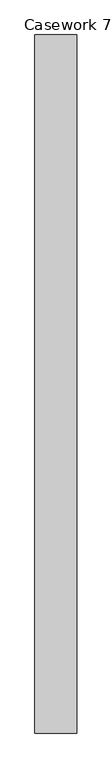
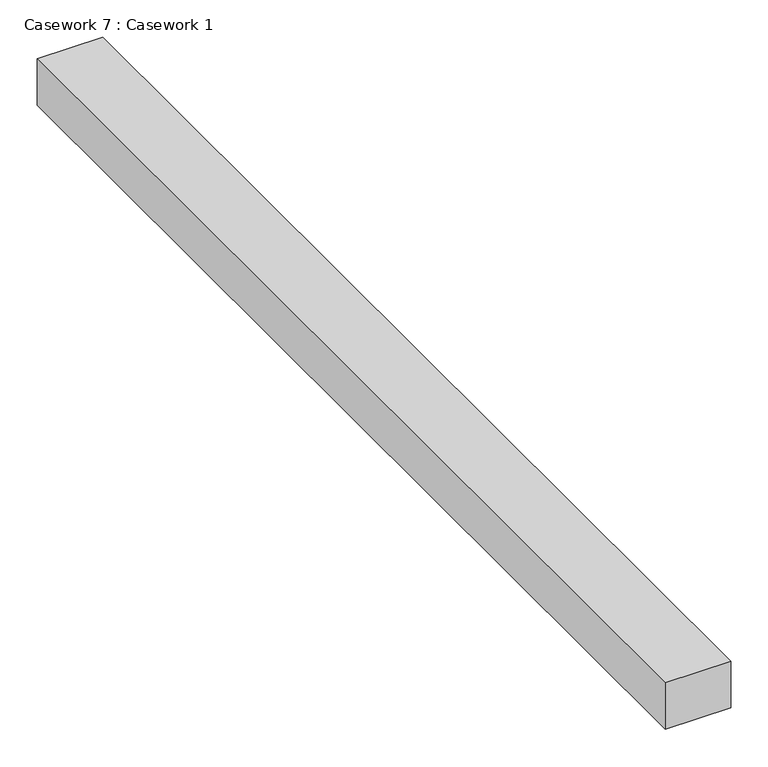
"""IFC4 building model written with IfcOpenShell, lengths in millimetres: furniture geometry, Casework 7 : Casework 1."""

from ifc_helpers import new_model, si_unit, frame, origin, place, context, project, spatial, polyline, outline, extrude, source, transform, mapped, element, save


def casework_7_casework_1_d1433357(model_context):
    return source(origin(), model_context, "Body", "SweptSolid", [
        extrude(outline(polyline([(7833.7559589, 14787.9496924), (7833.7559589, 13098.8496924), (7732.1559589, 13098.8496924), (7732.1559589, 14787.9496924), (7833.7559589, 14787.9496924)])), frame((0.0, 0.0, 3581.4), z_axis=(0.0, 0.0, 1.0), x_axis=(1.0, 0.0, 0.0)), (0.0, 0.0, 1.0), 76.2),
    ])


if __name__ == "__main__":
    model = new_model("IFC4")
    model_context = context("Model", 3, world=origin())
    ifc_project = project(units=[si_unit("LENGTHUNIT", "METRE", prefix="MILLI")], contexts=[model_context])
    site = spatial("IfcSite", under=ifc_project)
    building = spatial("IfcBuilding", under=site)
    placement = place(None, origin())
    casework_7_casework_1_shape = casework_7_casework_1_d1433357(model_context)
    element("IfcFurniture", 1, ObjectType="Casework 7 : Casework 1", at=placement, inside=building, context=model_context, shape_type="MappedRepresentation", body=[
        mapped(casework_7_casework_1_shape, transform((0.0, 0.0, 0.0), x_axis=(1.0, 0.0, 0.0), y_axis=(0.0, 1.0, 0.0), z_axis=(0.0, 0.0, 1.0))),
    ])
    save(model, "model.ifc")

# Revit data of these elements
# Element 1 (IfcFurniture, "Casework 7 : Casework 1")
#   Materials on its faces: "Clad - White"
# Materials
#   "Clad - White": class "Wood", colour RGB 242 242 238, transparency 0, Cost = 0
